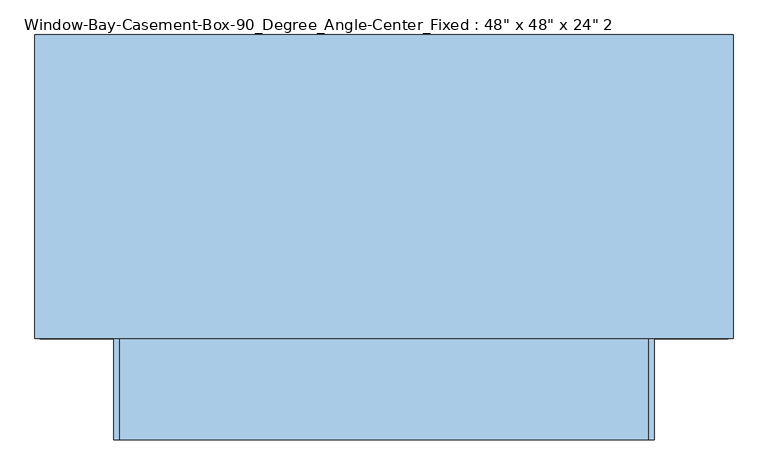
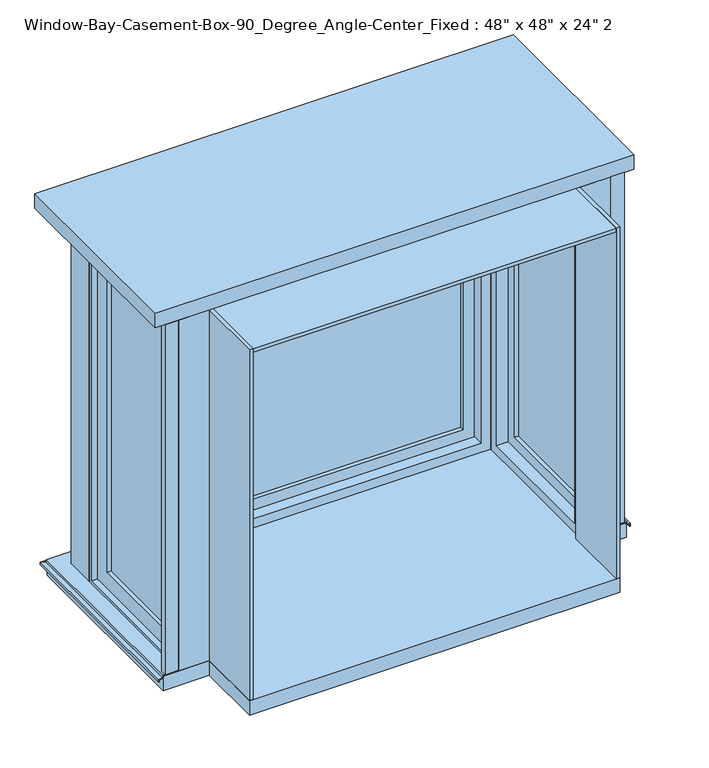
"""IFC4 building model written with IfcOpenShell, lengths in millimetres: window geometry."""

from ifc_helpers import new_model, si_unit, frame, origin, place, context, project, spatial, polyline, outline, extrude, faceted_brep, source, transform, mapped, element, save


def window_4fde904e(model_context):
    return source(origin(), model_context, "Body", "SolidModel", [
        extrude(outline(polyline([(-711.2, 114.3), (-755.65, 114.3), (-755.65, 133.35), (-711.2, 133.35), (-711.2, 114.3)])), frame((0.0, 0.0, 663.1486341), z_axis=(0.0, 0.0, 1.0), x_axis=(1.0, 0.0, 0.0)), (0.0, 0.0, 1.0), 1216.4513659),
        extrude(outline(polyline([(755.65, 114.3), (711.2, 114.3), (711.2, 133.35), (755.65, 133.35), (755.65, 114.3)])), frame((0.0, 0.0, 663.1486341), z_axis=(0.0, 0.0, 1.0), x_axis=(1.0, 0.0, 0.0)), (0.0, 0.0, 1.0), 1216.4513659),
        faceted_brep([(-762.0, 114.3, 653.0697935), (-762.0, 114.3, 660.4), (-711.2, 114.3, 660.4), (-711.2, 114.3, 663.1486341), (-763.397, 114.3, 663.1486341), (-763.397, 114.3, 654.4483503), (-776.097, 114.3, 652.2089977), (-776.097, 114.3, 643.2668038), (-772.1346, 114.3, 643.2668038), (-772.1346, 114.3, 644.7270038), (-774.4968, 114.3, 644.7270038), (-774.4968, 114.3, 650.8662705), (762.0, 114.3, 653.0697935), (774.4968, 114.3, 650.8662705), (774.4968, 114.3, 644.7270038), (772.1346, 114.3, 644.7270038), (772.1346, 114.3, 643.2668038), (776.097, 114.3, 643.2668038), (776.097, 114.3, 652.2089977), (763.397, 114.3, 654.4483503), (763.397, 114.3, 663.1486341), (711.2, 114.3, 663.1486341), (711.2, 114.3, 660.4), (762.0, 114.3, 660.4), (-762.0, 774.7, 653.0697935), (-762.0, 774.7, 660.4), (762.0, 774.7, 660.4), (711.2, 723.9, 660.4), (-711.2, 723.9, 660.4), (-711.2, 723.9, 663.1486341), (711.2, 723.9, 663.1486341), (763.397, 776.097, 663.1486341), (-763.397, 776.097, 663.1486341), (-763.397, 776.097, 654.4483503), (-776.097, 788.797, 652.2089977), (-776.097, 788.797, 643.2668038), (776.097, 788.797, 643.2668038), (772.1346, 784.8346, 643.2668038), (-772.1346, 784.8346, 643.2668038), (-772.1346, 784.8346, 644.7270038), (772.1346, 784.8346, 644.7270038), (774.4968, 787.1968, 644.7270038), (-774.4968, 787.1968, 644.7270038), (-774.4968, 787.1968, 650.8662705), (762.0, 774.7, 653.0697935), (763.397, 776.097, 654.4483503), (776.097, 788.797, 652.2089977), (774.4968, 787.1968, 650.8662705)], [[[0, 1, 2, 3, 4, 5, 6, 7, 8, 9, 10, 11]], [[12, 13, 14, 15, 16, 17, 18, 19, 20, 21, 22, 23]], [[1, 0, 24, 25]], [[2, 1, 25, 26, 23, 22, 27, 28]], [[3, 2, 28, 29]], [[4, 3, 29, 30, 21, 20, 31, 32]], [[5, 4, 32, 33]], [[6, 5, 33, 34]], [[7, 6, 34, 35]], [[8, 7, 35, 36, 17, 16, 37, 38]], [[9, 8, 38, 39]], [[10, 9, 39, 40, 15, 14, 41, 42]], [[11, 10, 42, 43]], [[0, 11, 43, 24]], [[25, 24, 44, 26]], [[29, 28, 27, 30]], [[33, 32, 31, 45]], [[34, 33, 45, 46]], [[35, 34, 46, 36]], [[39, 38, 37, 40]], [[43, 42, 41, 47]], [[24, 43, 47, 44]], [[26, 44, 12, 23]], [[30, 27, 22, 21]], [[45, 31, 20, 19]], [[46, 45, 19, 18]], [[36, 46, 18, 17]], [[40, 37, 16, 15]], [[47, 41, 14, 13]], [[44, 47, 13, 12]]]),
        extrude(outline(polyline([(762.0, 774.7), (762.0, 114.3), (609.6, 114.3), (609.6, -114.3), (-609.6, -114.3), (-609.6, 114.3), (-762.0, 114.3), (-762.0, 774.7), (762.0, 774.7)])), frame((0.0, 0.0, 609.6), z_axis=(0.0, 0.0, 1.0), x_axis=(1.0, 0.0, 0.0)), (0.0, 0.0, 1.0), 50.8),
        extrude(outline(polyline([(787.4, 800.1), (787.4, 114.3), (-787.4, 114.3), (-787.4, 800.1), (787.4, 800.1)])), frame((0.0, 0.0, 1879.6), z_axis=(0.0, 0.0, 1.0), x_axis=(1.0, 0.0, 0.0)), (0.0, 0.0, 1.0), 50.8),
        extrude(outline(polyline([(-609.6, 723.9), (-609.6, 622.3), (-711.2, 622.3), (-711.2, 723.9), (-609.6, 723.9)])), frame((0.0, 0.0, 660.4), z_axis=(0.0, 0.0, 1.0), x_axis=(1.0, 0.0, 0.0)), (0.0, 0.0, 1.0), 1219.2),
        extrude(outline(polyline([(711.2, 723.9), (711.2, 622.3), (609.6, 622.3), (609.6, 723.9), (711.2, 723.9)])), frame((0.0, 0.0, 660.4), z_axis=(0.0, 0.0, 1.0), x_axis=(1.0, 0.0, 0.0)), (0.0, 0.0, 1.0), 1219.2),
        faceted_brep([(596.9, 660.4, 673.1), (596.9, 723.9, 673.1), (-596.9, 723.9, 673.1), (-596.9, 660.4, 673.1), (577.85, 622.3, 692.15), (577.85, 660.4, 692.15), (-577.85, 660.4, 692.15), (-577.85, 622.3, 692.15), (609.6, 723.9, 660.4), (609.6, 622.3, 660.4), (-609.6, 622.3, 660.4), (-609.6, 723.9, 660.4), (-596.9, 723.9, 1866.9), (-596.9, 660.4, 1866.9), (-577.85, 660.4, 1847.85), (-577.85, 622.3, 1847.85), (-609.6, 622.3, 1879.6), (-609.6, 723.9, 1879.6), (596.9, 723.9, 1866.9), (596.9, 660.4, 1866.9), (577.85, 660.4, 1847.85), (577.85, 622.3, 1847.85), (609.6, 622.3, 1879.6), (609.6, 723.9, 1879.6)], [[[0, 1, 2, 3]], [[4, 5, 6, 7]], [[8, 9, 10, 11]], [[3, 2, 12, 13]], [[7, 6, 14, 15]], [[11, 10, 16, 17]], [[13, 12, 18, 19]], [[15, 14, 20, 21]], [[17, 16, 22, 23]], [[11, 17, 23, 8], [1, 18, 12, 2]], [[19, 18, 1, 0]], [[3, 13, 19, 0], [5, 20, 14, 6]], [[21, 20, 5, 4]], [[9, 22, 16, 10], [7, 15, 21, 4]], [[23, 22, 9, 8]]]),
        extrude(outline(polyline([(1866.9, -596.9), (673.1, -596.9), (673.1, 596.9), (1866.9, 596.9), (1866.9, -596.9)]), holes=[polyline([(1809.75, 539.75), (730.25, 539.75), (730.25, -539.75), (1809.75, -539.75), (1809.75, 539.75)])]), frame((0.0, 660.4, 0.0), z_axis=(0.0, 1.0, 0.0), x_axis=(0.0, 0.0, 1.0)), (0.0, 0.0, 1.0), 44.45),
        faceted_brep([(-609.6, 146.05, 1847.85), (-647.7, 146.05, 1847.85), (-647.7, 590.55, 1847.85), (-609.6, 590.55, 1847.85), (-711.2, 114.3, 1879.6), (-609.6, 114.3, 1879.6), (-609.6, 622.3, 1879.6), (-711.2, 622.3, 1879.6), (-647.7, 127.0, 1866.9), (-711.2, 127.0, 1866.9), (-711.2, 609.6, 1866.9), (-647.7, 609.6, 1866.9), (-647.7, 590.55, 692.15), (-609.6, 590.55, 692.15), (-609.6, 622.3, 660.4), (-711.2, 622.3, 660.4), (-711.2, 609.6, 673.1), (-647.7, 609.6, 673.1), (-647.7, 146.05, 692.15), (-609.6, 146.05, 692.15), (-609.6, 114.3, 660.4), (-711.2, 114.3, 660.4), (-711.2, 127.0, 673.1), (-647.7, 127.0, 673.1)], [[[0, 1, 2, 3]], [[4, 5, 6, 7]], [[8, 9, 10, 11]], [[3, 2, 12, 13]], [[7, 6, 14, 15]], [[11, 10, 16, 17]], [[13, 12, 18, 19]], [[15, 14, 20, 21]], [[17, 16, 22, 23]], [[11, 17, 23, 8], [1, 18, 12, 2]], [[19, 18, 1, 0]], [[5, 20, 14, 6], [3, 13, 19, 0]], [[21, 20, 5, 4]], [[7, 15, 21, 4], [9, 22, 16, 10]], [[23, 22, 9, 8]]]),
        extrude(outline(polyline([(609.6, 1866.9), (609.6, 673.1), (127.0, 673.1), (127.0, 1866.9), (609.6, 1866.9)]), holes=[polyline([(184.15, 1809.75), (184.15, 730.25), (552.45, 730.25), (552.45, 1809.75), (184.15, 1809.75)])]), frame((-692.15, 0.0, 0.0), z_axis=(1.0, 0.0, 0.0), x_axis=(0.0, 1.0, 0.0)), (0.0, 0.0, 1.0), 44.45),
        faceted_brep([(647.7, 146.05, 1847.85), (609.6, 146.05, 1847.85), (609.6, 590.55, 1847.85), (647.7, 590.55, 1847.85), (711.2, 127.0, 1866.9), (647.7, 127.0, 1866.9), (647.7, 609.6, 1866.9), (711.2, 609.6, 1866.9), (609.6, 114.3, 1879.6), (711.2, 114.3, 1879.6), (711.2, 622.3, 1879.6), (609.6, 622.3, 1879.6), (609.6, 590.55, 692.15), (647.7, 590.55, 692.15), (647.7, 609.6, 673.1), (711.2, 609.6, 673.1), (711.2, 622.3, 660.4), (609.6, 622.3, 660.4), (609.6, 146.05, 692.15), (647.7, 146.05, 692.15), (647.7, 127.0, 673.1), (711.2, 127.0, 673.1), (711.2, 114.3, 660.4), (609.6, 114.3, 660.4)], [[[0, 1, 2, 3]], [[4, 5, 6, 7]], [[8, 9, 10, 11]], [[3, 2, 12, 13]], [[7, 6, 14, 15]], [[11, 10, 16, 17]], [[13, 12, 18, 19]], [[15, 14, 20, 21]], [[17, 16, 22, 23]], [[11, 17, 23, 8], [1, 18, 12, 2]], [[19, 18, 1, 0]], [[5, 20, 14, 6], [3, 13, 19, 0]], [[21, 20, 5, 4]], [[9, 22, 16, 10], [7, 15, 21, 4]], [[23, 22, 9, 8]]]),
        extrude(outline(polyline([(609.6, 1866.9), (609.6, 673.1), (127.0, 673.1), (127.0, 1866.9), (609.6, 1866.9)]), holes=[polyline([(184.15, 1809.75), (184.15, 730.25), (552.45, 730.25), (552.45, 1809.75), (184.15, 1809.75)])]), frame((647.7, 0.0, 0.0), z_axis=(1.0, 0.0, 0.0), x_axis=(0.0, 1.0, 0.0)), (0.0, 0.0, 1.0), 44.45),
        extrude(outline(polyline([(539.75, 692.15), (539.75, 685.8), (-539.75, 685.8), (-539.75, 692.15), (539.75, 692.15)])), frame((0.0, 0.0, 730.25), z_axis=(0.0, 0.0, 1.0), x_axis=(1.0, 0.0, 0.0)), (0.0, 0.0, 1.0), 1079.5),
        extrude(outline(polyline([(539.75, 679.45), (539.75, 673.1), (-539.75, 673.1), (-539.75, 679.45), (539.75, 679.45)])), frame((0.0, 0.0, 730.25), z_axis=(0.0, 0.0, 1.0), x_axis=(1.0, 0.0, 0.0)), (0.0, 0.0, 1.0), 1079.5),
        extrude(outline(polyline([(-673.1, 552.45), (-673.1, 184.15), (-679.45, 184.15), (-679.45, 552.45), (-673.1, 552.45)])), frame((0.0, 0.0, 730.25), z_axis=(0.0, 0.0, 1.0), x_axis=(1.0, 0.0, 0.0)), (0.0, 0.0, 1.0), 1079.5),
        extrude(outline(polyline([(-660.4, 552.45), (-660.4, 184.15), (-666.75, 184.15), (-666.75, 552.45), (-660.4, 552.45)])), frame((0.0, 0.0, 730.25), z_axis=(0.0, 0.0, 1.0), x_axis=(1.0, 0.0, 0.0)), (0.0, 0.0, 1.0), 1079.5),
        extrude(outline(polyline([(679.45, 552.45), (679.45, 184.15), (673.1, 184.15), (673.1, 552.45), (679.45, 552.45)])), frame((0.0, 0.0, 730.25), z_axis=(0.0, 0.0, 1.0), x_axis=(1.0, 0.0, 0.0)), (0.0, 0.0, 1.0), 1079.5),
        extrude(outline(polyline([(666.75, 552.45), (666.75, 184.15), (660.4, 184.15), (660.4, 552.45), (666.75, 552.45)])), frame((0.0, 0.0, 730.25), z_axis=(0.0, 0.0, 1.0), x_axis=(1.0, 0.0, 0.0)), (0.0, 0.0, 1.0), 1079.5),
        faceted_brep([(711.2, 127.0, 1866.9), (647.7, 127.0, 1866.9), (647.7, 609.6, 1866.9), (711.2, 609.6, 1866.9), (609.6, 114.3, 1879.6), (711.2, 114.3, 1879.6), (711.2, 622.3, 1879.6), (609.6, 622.3, 1879.6), (647.7, 146.05, 1847.85), (609.6, 146.05, 1847.85), (609.6, 590.55, 1847.85), (647.7, 590.55, 1847.85), (647.7, 609.6, 673.1), (711.2, 609.6, 673.1), (711.2, 622.3, 660.4), (609.6, 622.3, 660.4), (609.6, 590.55, 692.15), (647.7, 590.55, 692.15), (647.7, 127.0, 673.1), (711.2, 127.0, 673.1), (711.2, 114.3, 660.4), (609.6, 114.3, 660.4), (609.6, 146.05, 692.15), (647.7, 146.05, 692.15)], [[[0, 1, 2, 3]], [[4, 5, 6, 7]], [[8, 9, 10, 11]], [[3, 2, 12, 13]], [[7, 6, 14, 15]], [[11, 10, 16, 17]], [[13, 12, 18, 19]], [[15, 14, 20, 21]], [[17, 16, 22, 23]], [[1, 18, 12, 2], [11, 17, 23, 8]], [[19, 18, 1, 0]], [[5, 20, 14, 6], [3, 13, 19, 0]], [[21, 20, 5, 4]], [[7, 15, 21, 4], [9, 22, 16, 10]], [[23, 22, 9, 8]]]),
        extrude(outline(polyline([(-596.9, 114.3), (-596.9, -114.3), (-609.6, -114.3), (-609.6, 114.3), (-596.9, 114.3)])), frame((0.0, 0.0, 660.4), z_axis=(0.0, 0.0, 1.0), x_axis=(1.0, 0.0, 0.0)), (0.0, 0.0, 1.0), 1219.2),
        extrude(outline(polyline([(596.9, 114.3), (609.6, 114.3), (609.6, -114.3), (596.9, -114.3), (596.9, 114.3)])), frame((0.0, 0.0, 660.4), z_axis=(0.0, 0.0, 1.0), x_axis=(1.0, 0.0, 0.0)), (0.0, 0.0, 1.0), 1219.2),
        extrude(outline(polyline([(596.9, -114.3), (-596.9, -114.3), (-596.9, 622.3), (596.9, 622.3), (596.9, -114.3)])), frame((0.0, 0.0, 1866.9), z_axis=(0.0, 0.0, 1.0), x_axis=(1.0, 0.0, 0.0)), (0.0, 0.0, 1.0), 12.7),
    ])


if __name__ == "__main__":
    model = new_model("IFC4")
    model_context = context("Model", 3, world=origin())
    ifc_project = project(units=[si_unit("LENGTHUNIT", "METRE", prefix="MILLI")], contexts=[model_context])
    site = spatial("IfcSite", under=ifc_project)
    building = spatial("IfcBuilding", under=site)
    placement = place(None, origin())
    window_shape = window_4fde904e(model_context)
    element("IfcWindow", 1, ObjectType="Window-Bay-Casement-Box-90_Degree_Angle-Center_Fixed : 48\" x 48\" x 24\" 2", at=placement, inside=building, context=model_context, shape_type="MappedRepresentation", body=[
        mapped(window_shape, transform((0.0, 0.0, 0.0), x_axis=(1.0, 0.0, 0.0), y_axis=(0.0, 1.0, 0.0), z_axis=(0.0, 0.0, 1.0))),
    ])
    save(model, "model.ifc")

# Revit data of these elements
# Type "Window-Bay-Casement-Box-90_Degree_Angle-Center_Fixed : 48\" x 48\" x 24\" 2"
#   Type Mark = "22"
#   Fire Rating = "0.5h"
#   Assembly Code = "B2020100"
#   Analytic Construction = "1/8 in Pilkington single glazing"
#   Width = 4' - 0"
#   Wall Thickness [instance default] = 0' - 6"
#   Visual Light Transmittance = 0.9
#   Trim Width = 4' - 8"
#   Trim Height = 4' - 0"
#   Thermal Resistance (R) = 1.5394 (h·ft²·°F)/BTU
#   Solar Heat Gain Coefficient = 0.86
#   Rough Width = 4' - 0 1/2"
#   Rough Height = 4' - 0 1/2"
#   Height 1 = 4' - 2"
#   Height = 4' - 0"
#   Heat Transfer Coefficient (U) = 0.6496 BTU/(h·ft²·°F)
#   Depth = 2' - 0"
#   Default Sill Height = 2' - 0"
#   Side Muntin Visibility = yes
#   Center Muntin Visibility = yes
#   Interior Trim Visibility [instance default] = yes
#   Exterior Trim Visibility [instance default] = yes
#   Side Muntin Pattern = Muntin Pattern_2x2 : Muntin Pattern_2x2
#   Center Muntin Pattern = Muntin Pattern_2x2 : Muntin Pattern_2x2
#   Interior Trim Material = Wood - Stained
#   Exterior Trim Material = Clad - White
#   Exterior Trim = element 393412
#   Interior Trim = Trim-Window-Interior-Flat : Picture Frame
#   Interior Frame Material = Wood - Stained
#   Glass Panel Material = Glass
#   Exterior Frame Material = Clad - White
#   Wall Closure = (empty or 0)
# Element 1 (IfcWindow, "Window-Bay-Casement-Box-90_Degree_Angle-Center_Fixed : 48\" x 48\" x 24\" 2")
#   Wall Thickness = 0' - 9"
#   Materials on its faces: "Clad - White", "Wood - Stained", "Glass"
# Materials
#   "Wood - Stained": class "Wood", colour RGB 224 178 126, transparency 0, Cost = 0
#   "Clad - White": class "Wood", colour RGB 242 242 238, transparency 0, Cost = 0
#   "Glass": class "Glass", colour RGB 0 128 192, transparency 0.75, Description = "Soda Lime Glass", Cost = 0
